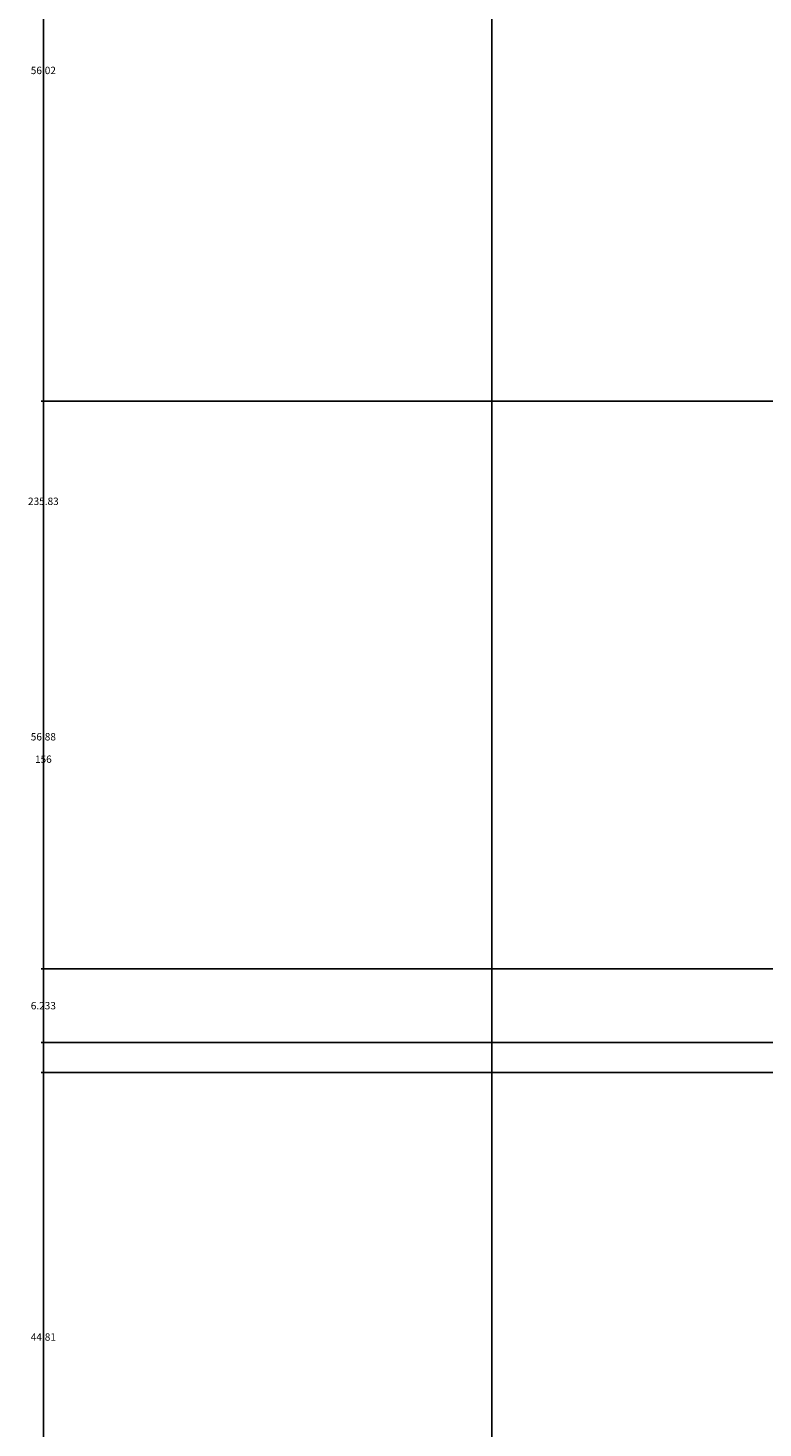
# Model space of a CAD drawing. Units: inches. Extents: x -13 to 809, y 112 to 656.
# Tile 5 of 55: x -13 to 49, y 328 to 446. Entities that reach past the tile are written whole.
import ezdxf

# ---------------------------------------------------------------- set-up
doc = ezdxf.new("R2010")
doc.units = ezdxf.units.IN
doc.header["$MEASUREMENT"] = 0
doc.layers.add('A-ANNO-DIMS', color=2, linetype='Continuous', lineweight=18)
doc.styles.get("Standard").update_dxf_attribs({"font": 'arial.ttf'})
doc.dimstyles.get("Standard").update_dxf_attribs({"dimtxt": 0.625, "dimasz": 0.18, "dimexe": 0.18, "dimexo": 0.0625, "dimgap": 0.09, "dimtad": 0, "dimtih": 1, "dimtoh": 1, "dimdec": 4, "dimzin": 0, "dimdsep": 46, "dimlunit": 4, "dimtxsty": 'Standard', "dimcen": 0.09, "dimadec": 0, "dimazin": 0, "dimtfac": 1, "dimtdec": 4, "dimtofl": 0, "dimtmove": 0, "dimatfit": 3, "dimfxl": 1, "dimtolj": 1, "dimtzin": 0, "dimarcsym": 0})

# ---------------------------------------------------------------- blocks, each defined once
blk = doc.blocks.new('*D22')
at = {"layer": 'A-ANNO-DIMS', "color": 0, "lineweight": -2, "transparency": 16777216}
for p, q in [((26.08, 210.58), (26.08, 655.96)), ((107.26, 510.58), (107.26, 655.96)), ((26.26, 655.78), (65.52, 655.78)), ((107.08, 655.78), (67.82, 655.78))]:
    blk.add_line(p, q, dxfattribs=at)
at = {"layer": 'A-ANNO-DIMS', "color": 0, "transparency": 16777216}
for points in [[(26.26, 655.81), (26.26, 655.75), (26.08, 655.78)], [(107.08, 655.81), (107.08, 655.75), (107.26, 655.78)]]:
    blk.add_solid(points, dxfattribs=at)
at = {"layer": 'Defpoints', "color": 0, "transparency": 16777216}
for p in [(107.26, 655.78), (107.26, 510.52), (26.08, 210.52)]:
    blk.add_point(p, dxfattribs=at)
at = {"layer": 'A-ANNO-DIMS', "color": 0, "transparency": 16777216, "insert": (66.67, 655.78), "char_height": 0.625, "attachment_point": 5}
blk.add_mtext('\\A1;81.18', dxfattribs=at)
blk = doc.blocks.new('*D34')
at = {"layer": 'A-ANNO-DIMS', "color": 0, "lineweight": -2, "transparency": 16777216}
for p, q in [((94.98, 462.52), (-12.1, 462.52)), ((-11.92, 462.34), (-11.92, 384.93)), ((-11.92, 306.7), (-11.92, 384.11)), ((94.98, 306.52), (-12.1, 306.52))]:
    blk.add_line(p, q, dxfattribs=at)
at = {"layer": 'A-ANNO-DIMS', "color": 0, "transparency": 16777216}
for points in [[(-11.95, 462.34), (-11.89, 462.34), (-11.92, 462.52)], [(-11.95, 306.7), (-11.89, 306.7), (-11.92, 306.52)]]:
    blk.add_solid(points, dxfattribs=at)
at = {"layer": 'Defpoints', "color": 0, "transparency": 16777216}
for p in [(-11.92, 462.52), (95.05, 462.52), (95.05, 306.52)]:
    blk.add_point(p, dxfattribs=at)
at = {"layer": 'A-ANNO-DIMS', "color": 0, "transparency": 16777216, "insert": (-11.92, 384.52), "char_height": 0.625, "attachment_point": 5}
blk.add_mtext('\\A1;156', dxfattribs=at)
blk = doc.blocks.new('*D39')
at = {"layer": 'A-ANNO-DIMS', "color": 0, "lineweight": -2, "transparency": 16777216}
for p, q in [((341.34, 524.28), (-12.1, 524.28)), ((-11.92, 524.1), (-11.92, 406.78)), ((-11.92, 288.63), (-11.92, 405.96)), ((341.34, 288.45), (-12.1, 288.45))]:
    blk.add_line(p, q, dxfattribs=at)
at = {"layer": 'A-ANNO-DIMS', "color": 0, "transparency": 16777216}
for points in [[(-11.95, 524.1), (-11.89, 524.1), (-11.92, 524.28)], [(-11.95, 288.63), (-11.89, 288.63), (-11.92, 288.45)]]:
    blk.add_solid(points, dxfattribs=at)
at = {"layer": 'Defpoints', "color": 0, "transparency": 16777216}
for p in [(-11.92, 524.28), (341.41, 524.28), (341.41, 288.45)]:
    blk.add_point(p, dxfattribs=at)
at = {"layer": 'A-ANNO-DIMS', "color": 0, "transparency": 16777216, "insert": (-11.92, 406.37), "char_height": 0.625, "attachment_point": 5}
blk.add_mtext('\\A1;235.83', dxfattribs=at)
blk = doc.blocks.new('*D41')
at = {"layer": 'A-ANNO-DIMS', "color": 0, "lineweight": -2, "transparency": 16777216}
for p, q in [((471.04, 357.98), (-12.1, 357.98)), ((-11.92, 357.8), (-11.92, 335.98)), ((-11.92, 313.35), (-11.92, 335.16)), ((471.04, 313.17), (-12.1, 313.17))]:
    blk.add_line(p, q, dxfattribs=at)
at = {"layer": 'A-ANNO-DIMS', "color": 0, "transparency": 16777216}
for points in [[(-11.95, 357.8), (-11.89, 357.8), (-11.92, 357.98)], [(-11.95, 313.35), (-11.89, 313.35), (-11.92, 313.17)]]:
    blk.add_solid(points, dxfattribs=at)
at = {"layer": 'Defpoints', "color": 0, "transparency": 16777216}
for p in [(-11.92, 357.98), (471.1, 357.98), (471.1, 313.17)]:
    blk.add_point(p, dxfattribs=at)
at = {"layer": 'A-ANNO-DIMS', "color": 0, "transparency": 16777216, "insert": (-11.92, 335.57), "char_height": 0.625, "attachment_point": 5}
blk.add_mtext('\\A1;44.81', dxfattribs=at)
blk = doc.blocks.new('*D42')
at = {"layer": 'A-ANNO-DIMS', "color": 0, "lineweight": -2, "transparency": 16777216}
for p, q in [((471.04, 414.86), (-12.1, 414.86)), ((-11.92, 414.68), (-11.92, 386.83)), ((-11.92, 358.16), (-11.92, 386.01)), ((471.04, 357.98), (-12.1, 357.98))]:
    blk.add_line(p, q, dxfattribs=at)
at = {"layer": 'A-ANNO-DIMS', "color": 0, "transparency": 16777216}
for points in [[(-11.95, 414.68), (-11.89, 414.68), (-11.92, 414.86)], [(-11.95, 358.16), (-11.89, 358.16), (-11.92, 357.98)]]:
    blk.add_solid(points, dxfattribs=at)
at = {"layer": 'Defpoints', "color": 0, "transparency": 16777216}
for p in [(-11.92, 414.86), (471.1, 414.86), (471.1, 357.98)]:
    blk.add_point(p, dxfattribs=at)
at = {"layer": 'A-ANNO-DIMS', "color": 0, "transparency": 16777216, "insert": (-11.92, 386.42), "char_height": 0.625, "attachment_point": 5}
blk.add_mtext('\\A1;56.88', dxfattribs=at)
blk = doc.blocks.new('*D43')
at = {"layer": 'A-ANNO-DIMS', "color": 0, "lineweight": -2, "transparency": 16777216}
for p, q in [((471.04, 470.88), (-12.1, 470.88)), ((-11.92, 470.7), (-11.92, 443.28)), ((-11.92, 415.04), (-11.92, 442.46)), ((471.04, 414.86), (-12.1, 414.86))]:
    blk.add_line(p, q, dxfattribs=at)
at = {"layer": 'A-ANNO-DIMS', "color": 0, "transparency": 16777216}
for points in [[(-11.95, 470.7), (-11.89, 470.7), (-11.92, 470.88)], [(-11.95, 415.04), (-11.89, 415.04), (-11.92, 414.86)]]:
    blk.add_solid(points, dxfattribs=at)
at = {"layer": 'Defpoints', "color": 0, "transparency": 16777216}
for p in [(-11.92, 470.88), (471.1, 470.88), (471.1, 414.86)]:
    blk.add_point(p, dxfattribs=at)
at = {"layer": 'A-ANNO-DIMS', "color": 0, "transparency": 16777216, "insert": (-11.92, 442.87), "char_height": 0.625, "attachment_point": 5}
blk.add_mtext('\\A1;56.02', dxfattribs=at)
blk = doc.blocks.new('*D114')
at = {"layer": 'A-ANNO-DIMS', "color": 0, "lineweight": -2, "transparency": 16777216}
for p, q in [((112.98, 366.75), (-12.1, 366.75)), ((-11.92, 366.57), (-11.92, 364.05)), ((-11.92, 360.7), (-11.92, 363.23)), ((112.98, 360.52), (-12.1, 360.52))]:
    blk.add_line(p, q, dxfattribs=at)
at = {"layer": 'A-ANNO-DIMS', "color": 0, "transparency": 16777216}
for points in [[(-11.95, 366.57), (-11.89, 366.57), (-11.92, 366.75)], [(-11.95, 360.7), (-11.89, 360.7), (-11.92, 360.52)]]:
    blk.add_solid(points, dxfattribs=at)
at = {"layer": 'Defpoints', "color": 0, "transparency": 16777216}
for p in [(113.05, 366.75), (-11.92, 360.52), (113.05, 360.52)]:
    blk.add_point(p, dxfattribs=at)
at = {"layer": 'A-ANNO-DIMS', "color": 0, "transparency": 16777216, "insert": (-11.92, 363.64), "char_height": 0.625, "attachment_point": 5}
blk.add_mtext('\\A1;6.233', dxfattribs=at)

msp = doc.modelspace()

# ---------------------------------------------------------------- dimensions: what is measured, and where the dimension line sits
at = {"layer": 'A-ANNO-DIMS'}
dim = msp.add_linear_dim(base=(107.2588, 655.7828), p1=(26.0809, 210.5199), p2=(107.2588, 510.5199), dimstyle='Standard', override={"dimdec": 2, "dimlfac": 1, "dimrnd": 0, "dimzin": 0, "dimdsep": 46, "dimlunit": 2}, dxfattribs=at)
dim.commit()
dim.dimension.update_dxf_attribs({"geometry": '*D22', "text_midpoint": (66.6698, 655.7828)})
for base, p1, p2, override, picture, middle in [((-11.9191, 524.281), (341.4072, 288.4508), (341.4072, 524.281), {"dimdec": 2, "dimlfac": 1, "dimrnd": 0, "dimzin": 0, "dimdsep": 46, "dimlunit": 2}, '*D39', (-11.9191, 406.3659)), ((-11.9191, 470.8765), (471.0998, 414.8594), (471.0998, 470.8765), {"dimdec": 2, "dimlfac": 1, "dimrnd": 0, "dimzin": 0, "dimdsep": 46, "dimlunit": 2}, '*D43', (-11.9191, 442.8679)), ((-11.9191, 462.5199), (95.0469, 306.5199), (95.0469, 462.5199), {"dimdec": 0, "dimlfac": 1, "dimrnd": 0, "dimzin": 0, "dimdsep": 46, "dimlunit": 2}, '*D34', (-11.9191, 384.5199)), ((-11.9191, 414.8594), (471.0998, 357.9804), (471.0998, 414.8594), {"dimdec": 2, "dimlfac": 1, "dimrnd": 0, "dimzin": 0, "dimdsep": 46, "dimlunit": 2}, '*D42', (-11.9191, 386.4199)), ((-11.9191, 360.5199), (113.0469, 366.753), (113.0469, 360.5199), {"dimdec": 3, "dimlfac": 1, "dimrnd": 0, "dimzin": 0, "dimdsep": 46, "dimlunit": 2}, '*D114', (-11.9191, 363.6364)), ((-11.9191, 357.9804), (471.0998, 313.1667), (471.0998, 357.9804), {"dimdec": 2, "dimlfac": 1, "dimrnd": 0, "dimzin": 0, "dimdsep": 46, "dimlunit": 2}, '*D41', (-11.9191, 335.5735))]:
    dim = msp.add_linear_dim(base=base, p1=p1, p2=p2, angle=90, dimstyle='Standard', override=override, dxfattribs=at)
    dim.commit()
    dim.dimension.update_dxf_attribs({"geometry": picture, "text_midpoint": middle})

doc.saveas('drawing.dxf')
